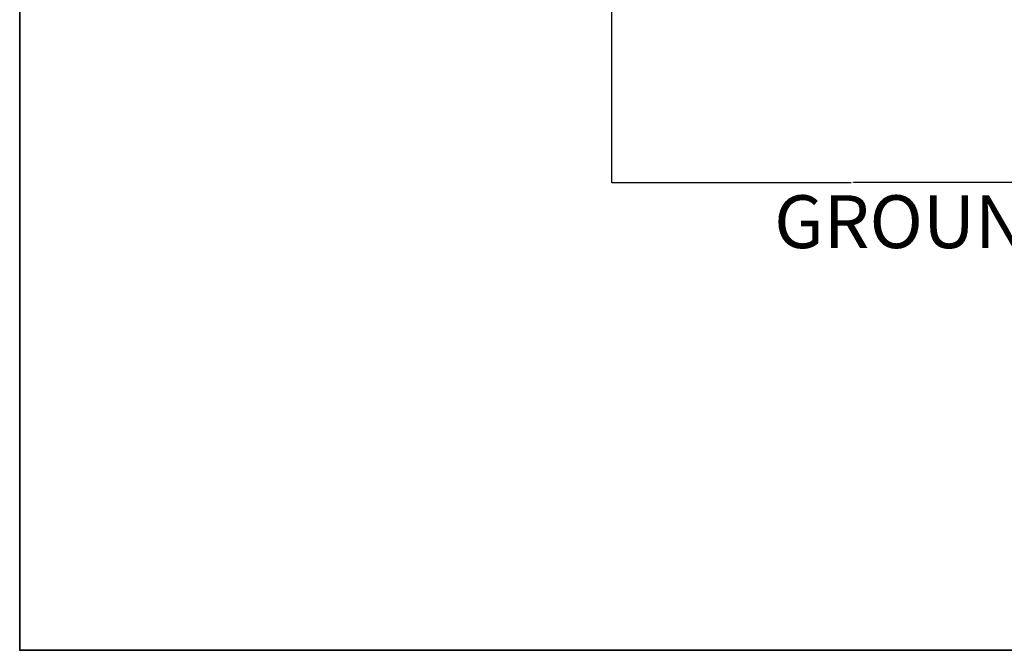
# Model space of a CAD drawing. Units: inches. Extents: x 2067 to 3463, y 1605 to 2723.
# Tile 1 of 10: x 2067 to 2403, y 1605 to 1820. Entities that reach past the tile are written whole.
import ezdxf

# ---------------------------------------------------------------- set-up
doc = ezdxf.new("R2010")
doc.units = ezdxf.units.IN
for name, color, linetype, lineweight in [('A-ANNO-DIMS', 2, 'Continuous', 18), ('A-ANNO-TEXT', 7, 'Continuous', 35), ('A-ANNO-TTLB', 7, 'Continuous', 35)]:
    doc.layers.add(name, color=color, linetype=linetype, lineweight=lineweight)
doc.styles.get("Standard").update_dxf_attribs({"font": 'arial.ttf'})
doc.dimstyles.get("Standard").update_dxf_attribs({"dimtxt": 0.18, "dimasz": 0.18, "dimexe": 0.18, "dimexo": 0.0625, "dimgap": 0.09, "dimtad": 0, "dimtih": 1, "dimtoh": 1, "dimdec": 4, "dimzin": 0, "dimdsep": 46, "dimtxsty": 'Standard', "dimcen": 0.09, "dimadec": 0, "dimazin": 0, "dimtfac": 1, "dimtdec": 4, "dimtofl": 0, "dimtmove": 0, "dimatfit": 3, "dimfxl": 1, "dimtolj": 1, "dimtzin": 0, "dimarcsym": 0})

# ---------------------------------------------------------------- blocks, each defined once
blk = doc.blocks.new('*D36')
at = {"layer": 'A-ANNO-DIMS', "color": 0, "lineweight": -2, "transparency": 16777216}
for p, q in [((2268.95, 1852.15), (2268.95, 1764.75)), ((2433.25, 1806.19), (2433.25, 1764.75)), ((2269.13, 1764.93), (2350.71, 1764.93)), ((2433.07, 1764.93), (2351.49, 1764.93))]:
    blk.add_line(p, q, dxfattribs=at)
at = {"layer": 'A-ANNO-DIMS', "color": 0, "transparency": 16777216}
for points in [[(2269.13, 1764.96), (2269.13, 1764.9), (2268.95, 1764.93)], [(2433.07, 1764.96), (2433.07, 1764.9), (2433.25, 1764.93)]]:
    blk.add_solid(points, dxfattribs=at)
at = {"layer": 'Defpoints', "color": 0, "transparency": 16777216}
for p in [(2268.95, 1852.22), (2433.25, 1806.25), (2433.25, 1764.93)]:
    blk.add_point(p, dxfattribs=at)
at = {"layer": 'A-ANNO-DIMS', "color": 0, "transparency": 16777216, "insert": (2351.1, 1764.93), "char_height": 0.18, "attachment_point": 5}
blk.add_mtext('\\A1;164.3', dxfattribs=at)

msp = doc.modelspace()

# ---------------------------------------------------------------- linework, layer by layer
at = {"layer": 'A-ANNO-TTLB'}
msp.add_lwpolyline([(2067.2624, 2722.6321), (3463.3053, 2722.6321), (3463.3053, 1605.3918), (2067.2624, 1605.3918)], close=True, dxfattribs=at)

# ---------------------------------------------------------------- texts
at = {"layer": 'A-ANNO-TEXT', "insert": (2324.4644, 1760.5241), "char_height": 18, "attachment_point": 1}
msp.add_mtext_dynamic_manual_height_columns('GROUND FLOOR PLAN', width=395.878396, gutter_width=12.5, heights=[0], dxfattribs=at)

# ---------------------------------------------------------------- dimensions: what is measured, and where the dimension line sits
at = {"layer": 'A-ANNO-DIMS'}
dim = msp.add_linear_dim(base=(2433.2522, 1764.9309), p1=(2268.9477, 1852.2171), p2=(2433.2522, 1806.2527), dimstyle='Standard', override={"dimdec": 1, "dimlfac": 1, "dimrnd": 0, "dimzin": 0, "dimdsep": 46, "dimlunit": 2}, dxfattribs=at)
dim.commit()
dim.dimension.update_dxf_attribs({"geometry": '*D36', "text_midpoint": (2351.0999, 1764.9309)})

doc.saveas('drawing.dxf')
